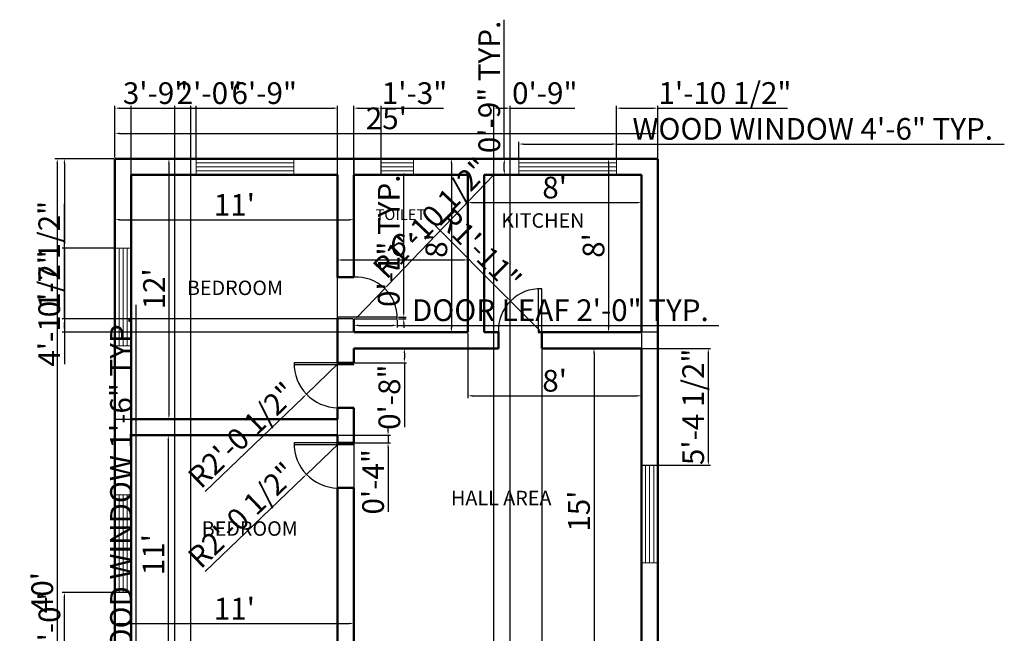
# Model space of a CAD drawing. Units: inches. Extents: x 2490 to 3058, y 1708 to 2351.
# Tile 2 of 2: x 2514 to 3058, y 2012 to 2351. Entities that reach past the tile are written whole.
import ezdxf

# ---------------------------------------------------------------- set-up
doc = ezdxf.new("R2010")
doc.units = ezdxf.units.IN
for name, color, linetype, lineweight in [('A-ANNO-DIMS', 2, 'Continuous', 18), ('A-AREA-IDEN', 7, 'Continuous', 25), ('A-DOOR', 3, 'Continuous', 25), ('A-GLAZ', 4, 'Continuous', 18), ('A-WALL', 7, 'Continuous', 50)]:
    doc.layers.add(name, color=color, linetype=linetype, lineweight=lineweight)
doc.styles.get("Standard").update_dxf_attribs({"font": 'arial.ttf'})
doc.dimstyles.new('ISO-25', dxfattribs={"dimtxt": 12, "dimasz": 2.5, "dimexe": 1.25, "dimexo": 0.625, "dimtad": 1, "dimdec": 1, "dimlunit": 3, "dimtxsty": 'Standard', "dimcen": 2.5, "dimadec": 0, "dimazin": 0, "dimtfac": 1, "dimtdec": 1, "dimtmove": 0, "dimatfit": 3, "dimfxl": 1, "dimarcsym": 0})

# ---------------------------------------------------------------- blocks, each defined once
blk = doc.blocks.new('*D1')
at = {"layer": 'A-ANNO-DIMS', "color": 0, "lineweight": -2, "transparency": 16777216}
for p, q in [((2567.47, 2274.57), (2597.88, 2274.57)), ((2596.63, 2272.07), (2596.63, 2133.07)), ((2567.47, 2130.57), (2597.88, 2130.57))]:
    blk.add_line(p, q, dxfattribs=at)
at = {"layer": 'A-ANNO-DIMS', "color": 0, "transparency": 16777216}
for points in [[(2596.21, 2272.07), (2597.04, 2272.07), (2596.63, 2274.57)], [(2596.21, 2133.07), (2597.04, 2133.07), (2596.63, 2130.57)]]:
    blk.add_solid(points, dxfattribs=at)
at = {"layer": 'Defpoints', "color": 0, "transparency": 16777216}
for p in [(2566.85, 2274.57), (2566.85, 2130.57), (2596.63, 2130.57)]:
    blk.add_point(p, dxfattribs=at)
at = {"layer": 'A-ANNO-DIMS', "color": 0, "transparency": 16777216, "insert": (2589.98, 2202.57), "char_height": 12, "attachment_point": 5, "rotation": 90}
blk.add_mtext("12'", dxfattribs=at)
blk = doc.blocks.new('*D2')
at = {"layer": 'A-ANNO-DIMS', "color": 0, "lineweight": -2, "transparency": 16777216}
for p, q in [((2566.85, 2273.95), (2566.85, 2239.59)), ((2698.85, 2273.95), (2698.85, 2239.59)), ((2569.35, 2240.84), (2696.35, 2240.84))]:
    blk.add_line(p, q, dxfattribs=at)
at = {"layer": 'A-ANNO-DIMS', "color": 0, "transparency": 16777216}
for points in [[(2569.35, 2241.26), (2569.35, 2240.42), (2566.85, 2240.84)], [(2696.35, 2241.26), (2696.35, 2240.42), (2698.85, 2240.84)]]:
    blk.add_solid(points, dxfattribs=at)
at = {"layer": 'Defpoints', "color": 0, "transparency": 16777216}
for p in [(2566.85, 2274.57), (2698.85, 2274.57), (2698.85, 2240.84)]:
    blk.add_point(p, dxfattribs=at)
at = {"layer": 'A-ANNO-DIMS', "color": 0, "transparency": 16777216, "insert": (2632.85, 2247.49), "char_height": 12, "attachment_point": 5}
blk.add_mtext("11'", dxfattribs=at)
blk = doc.blocks.new('*D3')
at = {"layer": 'A-ANNO-DIMS', "color": 0, "lineweight": -2, "transparency": 16777216}
for p, q in [((2689.85, 2209.6), (2689.85, 2219.81)), ((2692.35, 2218.56), (2759.35, 2218.56)), ((2761.85, 2209.6), (2761.85, 2219.81))]:
    blk.add_line(p, q, dxfattribs=at)
at = {"layer": 'A-ANNO-DIMS', "color": 0, "transparency": 16777216}
for points in [[(2692.35, 2218.98), (2692.35, 2218.14), (2689.85, 2218.56)], [(2759.35, 2218.98), (2759.35, 2218.14), (2761.85, 2218.56)]]:
    blk.add_solid(points, dxfattribs=at)
at = {"layer": 'Defpoints', "color": 0, "transparency": 16777216}
for p in [(2761.85, 2218.56), (2689.85, 2208.98), (2761.85, 2208.98)]:
    blk.add_point(p, dxfattribs=at)
at = {"layer": 'A-ANNO-DIMS', "color": 0, "transparency": 16777216, "insert": (2725.85, 2225.31), "char_height": 12, "attachment_point": 5}
blk.add_mtext("6'", dxfattribs=at)
blk = doc.blocks.new('*D4')
at = {"layer": 'A-ANNO-DIMS', "color": 0, "lineweight": -2, "transparency": 16777216}
for p, q in [((2699.47, 2274.57), (2754.03, 2274.57)), ((2752.78, 2272.07), (2752.78, 2181.07)), ((2699.47, 2178.57), (2754.03, 2178.57))]:
    blk.add_line(p, q, dxfattribs=at)
at = {"layer": 'A-ANNO-DIMS', "color": 0, "transparency": 16777216}
for points in [[(2752.37, 2272.07), (2753.2, 2272.07), (2752.78, 2274.57)], [(2752.37, 2181.07), (2753.2, 2181.07), (2752.78, 2178.57)]]:
    blk.add_solid(points, dxfattribs=at)
at = {"layer": 'Defpoints', "color": 0, "transparency": 16777216}
for p in [(2698.85, 2274.57), (2698.85, 2178.57), (2752.78, 2178.57)]:
    blk.add_point(p, dxfattribs=at)
at = {"layer": 'A-ANNO-DIMS', "color": 0, "transparency": 16777216, "insert": (2746.03, 2226.57), "char_height": 12, "attachment_point": 5, "rotation": 90}
blk.add_mtext("8'", dxfattribs=at)
blk = doc.blocks.new('*D5')
at = {"layer": 'A-ANNO-DIMS', "color": 0, "lineweight": -2, "transparency": 16777216}
for p, q in [((2761.85, 2264.95), (2761.85, 2249.05)), ((2857.85, 2264.95), (2857.85, 2249.05)), ((2764.35, 2250.3), (2855.35, 2250.3))]:
    blk.add_line(p, q, dxfattribs=at)
at = {"layer": 'A-ANNO-DIMS', "color": 0, "transparency": 16777216}
for points in [[(2764.35, 2250.71), (2764.35, 2249.88), (2761.85, 2250.3)], [(2855.35, 2250.71), (2855.35, 2249.88), (2857.85, 2250.3)]]:
    blk.add_solid(points, dxfattribs=at)
at = {"layer": 'Defpoints', "color": 0, "transparency": 16777216}
for p in [(2761.85, 2265.57), (2857.85, 2265.57), (2857.85, 2250.3)]:
    blk.add_point(p, dxfattribs=at)
at = {"layer": 'A-ANNO-DIMS', "color": 0, "transparency": 16777216, "insert": (2809.85, 2257.05), "char_height": 12, "attachment_point": 5}
blk.add_mtext("8'", dxfattribs=at)
blk = doc.blocks.new('*D6')
at = {"layer": 'A-ANNO-DIMS', "color": 0, "lineweight": -2, "transparency": 16777216}
for p, q in [((2866.22, 2274.57), (2838.4, 2274.57)), ((2839.65, 2272.07), (2839.65, 2181.07)), ((2866.22, 2178.57), (2838.4, 2178.57))]:
    blk.add_line(p, q, dxfattribs=at)
at = {"layer": 'A-ANNO-DIMS', "color": 0, "transparency": 16777216}
for points in [[(2839.24, 2272.07), (2840.07, 2272.07), (2839.65, 2274.57)], [(2839.24, 2181.07), (2840.07, 2181.07), (2839.65, 2178.57)]]:
    blk.add_solid(points, dxfattribs=at)
at = {"layer": 'Defpoints', "color": 0, "transparency": 16777216}
for p in [(2866.85, 2274.57), (2839.65, 2178.57), (2866.85, 2178.57)]:
    blk.add_point(p, dxfattribs=at)
at = {"layer": 'A-ANNO-DIMS', "color": 0, "transparency": 16777216, "insert": (2832.9, 2226.57), "char_height": 12, "attachment_point": 5, "rotation": 90}
blk.add_mtext("8'", dxfattribs=at)
blk = doc.blocks.new('*D7')
at = {"layer": 'A-ANNO-DIMS', "color": 0, "lineweight": -2, "transparency": 16777216}
for p, q in [((2597.25, 2121.57), (2595.04, 2121.57)), ((2596.29, 2119.07), (2596.29, 1992.07)), ((2597.25, 1989.57), (2595.04, 1989.57))]:
    blk.add_line(p, q, dxfattribs=at)
at = {"layer": 'A-ANNO-DIMS', "color": 0, "transparency": 16777216}
for points in [[(2595.88, 2119.07), (2596.71, 2119.07), (2596.29, 2121.57)], [(2595.88, 1992.07), (2596.71, 1992.07), (2596.29, 1989.57)]]:
    blk.add_solid(points, dxfattribs=at)
at = {"layer": 'Defpoints', "color": 0, "transparency": 16777216}
for p in [(2597.88, 2121.57), (2596.29, 1989.57), (2597.88, 1989.57)]:
    blk.add_point(p, dxfattribs=at)
at = {"layer": 'A-ANNO-DIMS', "color": 0, "transparency": 16777216, "insert": (2589.64, 2055.57), "char_height": 12, "attachment_point": 5, "rotation": 90}
blk.add_mtext("11'", dxfattribs=at)
blk = doc.blocks.new('*D8')
at = {"layer": 'A-ANNO-DIMS', "color": 0, "lineweight": -2, "transparency": 16777216}
for p, q in [((2566.85, 2120.95), (2566.85, 2016.22)), ((2698.85, 2120.95), (2698.85, 2016.22)), ((2569.35, 2017.47), (2696.35, 2017.47))]:
    blk.add_line(p, q, dxfattribs=at)
at = {"layer": 'A-ANNO-DIMS', "color": 0, "transparency": 16777216}
for points in [[(2569.35, 2017.89), (2569.35, 2017.05), (2566.85, 2017.47)], [(2696.35, 2017.89), (2696.35, 2017.05), (2698.85, 2017.47)]]:
    blk.add_solid(points, dxfattribs=at)
at = {"layer": 'Defpoints', "color": 0, "transparency": 16777216}
for p in [(2566.85, 2121.57), (2698.85, 2121.57), (2698.85, 2017.47)]:
    blk.add_point(p, dxfattribs=at)
at = {"layer": 'A-ANNO-DIMS', "color": 0, "transparency": 16777216, "insert": (2632.85, 2024.12), "char_height": 12, "attachment_point": 5}
blk.add_mtext("11'", dxfattribs=at)
blk = doc.blocks.new('*D14')
at = {"layer": 'A-ANNO-DIMS', "color": 0, "lineweight": -2, "transparency": 16777216}
for p, q in [((2847.51, 2169.63), (2830.36, 2169.63)), ((2831.61, 2167.13), (2831.61, 1992.13)), ((2847.51, 1989.63), (2830.36, 1989.63))]:
    blk.add_line(p, q, dxfattribs=at)
at = {"layer": 'A-ANNO-DIMS', "color": 0, "transparency": 16777216}
for points in [[(2831.19, 2167.13), (2832.02, 2167.13), (2831.61, 2169.63)], [(2831.19, 1992.13), (2832.02, 1992.13), (2831.61, 1989.63)]]:
    blk.add_solid(points, dxfattribs=at)
at = {"layer": 'Defpoints', "color": 0, "transparency": 16777216}
for p in [(2848.13, 2169.63), (2831.61, 1989.63), (2848.13, 1989.63)]:
    blk.add_point(p, dxfattribs=at)
at = {"layer": 'A-ANNO-DIMS', "color": 0, "transparency": 16777216, "insert": (2824.86, 2079.63), "char_height": 12, "attachment_point": 5, "rotation": 90}
blk.add_mtext("15'", dxfattribs=at)
blk = doc.blocks.new('*D15')
at = {"layer": 'A-ANNO-DIMS', "color": 0, "lineweight": -2, "transparency": 16777216}
for p, q in [((2761.85, 2177.95), (2761.85, 2142.17)), ((2857.85, 2177.95), (2857.85, 2142.17)), ((2764.35, 2143.42), (2855.35, 2143.42))]:
    blk.add_line(p, q, dxfattribs=at)
at = {"layer": 'A-ANNO-DIMS', "color": 0, "transparency": 16777216}
for points in [[(2764.35, 2143.84), (2764.35, 2143.01), (2761.85, 2143.42)], [(2855.35, 2143.84), (2855.35, 2143.01), (2857.85, 2143.42)]]:
    blk.add_solid(points, dxfattribs=at)
at = {"layer": 'Defpoints', "color": 0, "transparency": 16777216}
for p in [(2761.85, 2178.57), (2857.85, 2178.57), (2857.85, 2143.42)]:
    blk.add_point(p, dxfattribs=at)
at = {"layer": 'A-ANNO-DIMS', "color": 0, "transparency": 16777216, "insert": (2809.85, 2150.17), "char_height": 12, "attachment_point": 5}
blk.add_mtext("8'", dxfattribs=at)
blk = doc.blocks.new('Window - Wood Frame 36 in. Wide plan')
for p, q in [((0, 6), (0, 0)), ((0, 4.5), (36, 4.5)), ((36, 6), (36, 0)), ((0, 3), (36, 3)), ((0, 1.5), (36, 1.5))]:
    blk.add_line(p, q)
blk = doc.blocks.new('*D21')
at = {"layer": 'A-ANNO-DIMS', "color": 0, "lineweight": -2, "transparency": 16777216}
for p, q in [((2566.85, 2275.2), (2566.85, 2289.82)), ((2569.35, 2288.57), (2864.35, 2288.57)), ((2866.85, 2275.2), (2866.85, 2289.82))]:
    blk.add_line(p, q, dxfattribs=at)
at = {"layer": 'A-ANNO-DIMS', "color": 0, "transparency": 16777216}
for points in [[(2569.35, 2288.99), (2569.35, 2288.16), (2566.85, 2288.57)], [(2864.35, 2288.99), (2864.35, 2288.16), (2866.85, 2288.57)]]:
    blk.add_solid(points, dxfattribs=at)
at = {"layer": 'Defpoints', "color": 0, "transparency": 16777216}
for p in [(2866.85, 2288.57), (2566.85, 2274.57), (2866.85, 2274.57)]:
    blk.add_point(p, dxfattribs=at)
at = {"layer": 'A-ANNO-DIMS', "color": 0, "transparency": 16777216, "insert": (2716.85, 2295.33), "char_height": 12, "attachment_point": 5}
blk.add_mtext("25'", dxfattribs=at)
blk = doc.blocks.new('*D22')
at = {"layer": 'A-ANNO-DIMS', "color": 0, "lineweight": -2, "transparency": 16777216}
for p, q in [((2566.22, 2274.57), (2533.68, 2274.57)), ((2534.93, 2272.07), (2534.93, 1797.07)), ((2566.22, 1794.57), (2533.68, 1794.57))]:
    blk.add_line(p, q, dxfattribs=at)
at = {"layer": 'A-ANNO-DIMS', "color": 0, "transparency": 16777216}
for points in [[(2534.51, 2272.07), (2535.35, 2272.07), (2534.93, 2274.57)], [(2534.51, 1797.07), (2535.35, 1797.07), (2534.93, 1794.57)]]:
    blk.add_solid(points, dxfattribs=at)
at = {"layer": 'Defpoints', "color": 0, "transparency": 16777216}
for p in [(2566.85, 2274.57), (2534.93, 1794.57), (2566.85, 1794.57)]:
    blk.add_point(p, dxfattribs=at)
at = {"layer": 'A-ANNO-DIMS', "color": 0, "transparency": 16777216, "insert": (2528.18, 2034.57), "char_height": 12, "attachment_point": 5, "rotation": 90}
blk.add_mtext("40'", dxfattribs=at)
blk = doc.blocks.new('DOOR-LEAF-24IN')
for p, q in [((24, 1), (0, 1)), ((0, 0), (24, 0)), ((24, 0), (24, 1))]:
    blk.add_line(p, q)
blk = doc.blocks.new('*D24')
at = {"layer": 'A-ANNO-DIMS', "color": 0, "lineweight": -2, "transparency": 16777216}
for p, q in [((2790.13, 2275.2), (2790.13, 2283.92)), ((2792.63, 2282.67), (2841.63, 2282.67)), ((2844.13, 2275.2), (2844.13, 2283.92)), ((2844.13, 2282.67), (3058.39, 2282.67))]:
    blk.add_line(p, q, dxfattribs=at)
at = {"layer": 'A-ANNO-DIMS', "color": 0, "transparency": 16777216}
for points in [[(2792.63, 2283.09), (2792.63, 2282.25), (2790.13, 2282.67)], [(2841.63, 2283.09), (2841.63, 2282.25), (2844.13, 2282.67)]]:
    blk.add_solid(points, dxfattribs=at)
at = {"layer": 'Defpoints', "color": 0, "transparency": 16777216}
for p in [(2844.13, 2282.67), (2790.13, 2274.57), (2844.13, 2274.57)]:
    blk.add_point(p, dxfattribs=at)
at = {"layer": 'A-ANNO-DIMS', "color": 0, "transparency": 16777216, "insert": (2952.51, 2289.5), "char_height": 12, "attachment_point": 5}
blk.add_mtext('WOOD WINDOW 4\'-6" TYP.', dxfattribs=at)
blk = doc.blocks.new('*D25')
at = {"layer": 'A-ANNO-DIMS', "color": 0, "lineweight": -2, "transparency": 16777216}
for p, q in [((2782.03, 2274.57), (2782.03, 2351.47)), ((2789.5, 2274.57), (2780.78, 2274.57)), ((2782.03, 2268.07), (2782.03, 2272.07)), ((2789.5, 2265.57), (2780.78, 2265.57))]:
    blk.add_line(p, q, dxfattribs=at)
at = {"layer": 'A-ANNO-DIMS', "color": 0, "transparency": 16777216}
for points in [[(2781.61, 2272.07), (2782.44, 2272.07), (2782.03, 2274.57)], [(2781.61, 2268.07), (2782.44, 2268.07), (2782.03, 2265.57)]]:
    blk.add_solid(points, dxfattribs=at)
at = {"layer": 'Defpoints', "color": 0, "transparency": 16777216}
for p in [(2782.03, 2274.57), (2790.13, 2274.57), (2790.13, 2265.57)]:
    blk.add_point(p, dxfattribs=at)
at = {"layer": 'A-ANNO-DIMS', "color": 0, "transparency": 16777216, "insert": (2775.28, 2314.27), "char_height": 12, "attachment_point": 5, "rotation": 90}
blk.add_mtext('0\'-9" TYP.', dxfattribs=at)
blk = doc.blocks.new('*D26')
at = {"layer": 'A-ANNO-DIMS', "color": 0, "lineweight": -2, "transparency": 16777216}
for p, q in [((2578.55, 1979.48), (2578.55, 2193.75)), ((2576.47, 1979.48), (2579.8, 1979.48)), ((2578.55, 1963.98), (2578.55, 1976.98)), ((2576.47, 1961.48), (2579.8, 1961.48))]:
    blk.add_line(p, q, dxfattribs=at)
at = {"layer": 'A-ANNO-DIMS', "color": 0, "transparency": 16777216}
for points in [[(2578.13, 1976.98), (2578.97, 1976.98), (2578.55, 1979.48)], [(2578.13, 1963.98), (2578.97, 1963.98), (2578.55, 1961.48)]]:
    blk.add_solid(points, dxfattribs=at)
at = {"layer": 'Defpoints', "color": 0, "transparency": 16777216}
for p in [(2575.85, 1979.48), (2578.55, 1979.48), (2575.85, 1961.48)]:
    blk.add_point(p, dxfattribs=at)
at = {"layer": 'A-ANNO-DIMS', "color": 0, "transparency": 16777216, "insert": (2571.72, 2087.86), "char_height": 12, "attachment_point": 5, "rotation": 90}
blk.add_mtext('WOOD WINDOW 1\'-6" TYP.', dxfattribs=at)
blk = doc.blocks.new('*D28')
at = {"layer": 'A-ANNO-DIMS', "color": 0, "lineweight": -2, "transparency": 16777216}
for p, q in [((2698.85, 2185.35), (2698.85, 2181.13)), ((2701.35, 2182.38), (2720.35, 2182.38)), ((2722.85, 2185.35), (2722.85, 2181.13)), ((2722.85, 2182.38), (2900.68, 2182.38))]:
    blk.add_line(p, q, dxfattribs=at)
at = {"layer": 'A-ANNO-DIMS', "color": 0, "transparency": 16777216}
for points in [[(2701.35, 2182.8), (2701.35, 2181.96), (2698.85, 2182.38)], [(2720.35, 2182.8), (2720.35, 2181.96), (2722.85, 2182.38)]]:
    blk.add_solid(points, dxfattribs=at)
at = {"layer": 'Defpoints', "color": 0, "transparency": 16777216}
for p in [(2698.85, 2185.98), (2722.85, 2185.98), (2722.85, 2182.38)]:
    blk.add_point(p, dxfattribs=at)
at = {"layer": 'A-ANNO-DIMS', "color": 0, "transparency": 16777216, "insert": (2813.01, 2189.21), "char_height": 12, "attachment_point": 5}
blk.add_mtext('DOOR LEAF 2\'-0" TYP.', dxfattribs=at)
blk = doc.blocks.new('*D29')
at = {"layer": 'A-ANNO-DIMS', "color": 0, "lineweight": -2, "transparency": 16777216}
for p, q in [((2726.45, 2189.48), (2726.45, 2266.37)), ((2723.47, 2186.98), (2727.7, 2186.98)), ((2723.47, 2185.98), (2727.7, 2185.98)), ((2726.45, 2185.98), (2726.45, 2186.98)), ((2726.45, 2183.48), (2726.45, 2180.98))]:
    blk.add_line(p, q, dxfattribs=at)
at = {"layer": 'A-ANNO-DIMS', "color": 0, "transparency": 16777216}
for points in [[(2726.03, 2189.48), (2726.87, 2189.48), (2726.45, 2186.98)], [(2726.03, 2183.48), (2726.87, 2183.48), (2726.45, 2185.98)]]:
    blk.add_solid(points, dxfattribs=at)
at = {"layer": 'Defpoints', "color": 0, "transparency": 16777216}
for p in [(2722.85, 2186.98), (2722.85, 2185.98), (2726.45, 2186.98)]:
    blk.add_point(p, dxfattribs=at)
at = {"layer": 'A-ANNO-DIMS', "color": 0, "transparency": 16777216, "insert": (2719.7, 2229.18), "char_height": 12, "attachment_point": 5, "rotation": 90}
blk.add_mtext('0\'-1" TYP.', dxfattribs=at)
blk = doc.blocks.new('*D33')
at = {"layer": 'A-ANNO-DIMS', "color": 0, "lineweight": -2, "transparency": 16777216}
for p, q in [((2608.85, 1990.2), (2608.85, 2303.77)), ((2611.35, 2302.52), (2687.35, 2302.52)), ((2689.85, 1990.2), (2689.85, 2303.77))]:
    blk.add_line(p, q, dxfattribs=at)
at = {"layer": 'A-ANNO-DIMS', "color": 0, "transparency": 16777216}
for points in [[(2611.35, 2302.94), (2611.35, 2302.1), (2608.85, 2302.52)], [(2687.35, 2302.94), (2687.35, 2302.1), (2689.85, 2302.52)]]:
    blk.add_solid(points, dxfattribs=at)
at = {"layer": 'Defpoints', "color": 0, "transparency": 16777216}
for p in [(2689.85, 2302.52), (2608.85, 1989.57), (2689.85, 1989.57)]:
    blk.add_point(p, dxfattribs=at)
at = {"layer": 'A-ANNO-DIMS', "color": 0, "transparency": 16777216, "insert": (2649.35, 2309.27), "char_height": 12, "attachment_point": 5}
blk.add_mtext('6\'-9"', dxfattribs=at)
blk = doc.blocks.new('*D34')
at = {"layer": 'A-ANNO-DIMS', "color": 0, "lineweight": -2, "transparency": 16777216}
for p, q in [((2698.85, 2266.2), (2698.85, 2303.77)), ((2701.35, 2302.52), (2711.41, 2302.52)), ((2713.91, 2266.2), (2713.91, 2303.77)), ((2713.91, 2302.52), (2748.42, 2302.52))]:
    blk.add_line(p, q, dxfattribs=at)
at = {"layer": 'A-ANNO-DIMS', "color": 0, "transparency": 16777216}
for points in [[(2701.35, 2302.94), (2701.35, 2302.1), (2698.85, 2302.52)], [(2711.41, 2302.94), (2711.41, 2302.1), (2713.91, 2302.52)]]:
    blk.add_solid(points, dxfattribs=at)
at = {"layer": 'Defpoints', "color": 0, "transparency": 16777216}
for p in [(2713.91, 2302.52), (2698.85, 2265.57), (2713.91, 2265.57)]:
    blk.add_point(p, dxfattribs=at)
at = {"layer": 'A-ANNO-DIMS', "color": 0, "transparency": 16777216, "insert": (2732.42, 2309.28), "char_height": 12, "attachment_point": 5}
blk.add_mtext('1\'-3"', dxfattribs=at)
blk = doc.blocks.new('*D35')
at = {"layer": 'A-ANNO-DIMS', "color": 0, "lineweight": -2, "transparency": 16777216}
for p, q in [((2844.13, 2275.2), (2844.13, 2303.77)), ((2846.63, 2302.52), (2864.35, 2302.52)), ((2866.85, 2275.2), (2866.85, 2303.77)), ((2866.85, 2302.52), (2938.65, 2302.52))]:
    blk.add_line(p, q, dxfattribs=at)
at = {"layer": 'A-ANNO-DIMS', "color": 0, "transparency": 16777216}
for points in [[(2846.63, 2302.94), (2846.63, 2302.1), (2844.13, 2302.52)], [(2864.35, 2302.94), (2864.35, 2302.1), (2866.85, 2302.52)]]:
    blk.add_solid(points, dxfattribs=at)
at = {"layer": 'Defpoints', "color": 0, "transparency": 16777216}
for p in [(2866.85, 2302.52), (2844.13, 2274.57), (2866.85, 2274.57)]:
    blk.add_point(p, dxfattribs=at)
at = {"layer": 'A-ANNO-DIMS', "color": 0, "transparency": 16777216, "insert": (2904, 2309.35), "char_height": 12, "attachment_point": 5}
blk.add_mtext('1\'-10 1/2"', dxfattribs=at)
blk = doc.blocks.new('*D36')
at = {"layer": 'A-ANNO-DIMS', "color": 0, "lineweight": -2, "transparency": 16777216}
for p, q in [((2802.74, 2168.95), (2802.74, 1718.25)), ((2857.85, 2168.95), (2857.85, 1718.25)), ((2805.24, 1719.5), (2855.35, 1719.5))]:
    blk.add_line(p, q, dxfattribs=at)
at = {"layer": 'A-ANNO-DIMS', "color": 0, "transparency": 16777216}
for points in [[(2805.24, 1719.92), (2805.24, 1719.08), (2802.74, 1719.5)], [(2855.35, 1719.92), (2855.35, 1719.08), (2857.85, 1719.5)]]:
    blk.add_solid(points, dxfattribs=at)
at = {"layer": 'Defpoints', "color": 0, "transparency": 16777216}
for p in [(2802.74, 2169.57), (2857.85, 2169.57), (2857.85, 1719.5)]:
    blk.add_point(p, dxfattribs=at)
at = {"layer": 'A-ANNO-DIMS', "color": 0, "transparency": 16777216, "insert": (2830.3, 1726.12), "char_height": 12, "attachment_point": 5}
blk.add_mtext('4\'-7"', dxfattribs=at)
blk = doc.blocks.new('*D37')
at = {"layer": 'A-ANNO-DIMS', "color": 0, "lineweight": -2, "transparency": 16777216}
for p, q in [((2538.9, 2185.98), (2538.9, 2249.59)), ((2698.22, 2185.98), (2537.65, 2185.98)), ((2538.9, 2181.07), (2538.9, 2183.48)), ((2698.22, 2178.57), (2537.65, 2178.57))]:
    blk.add_line(p, q, dxfattribs=at)
at = {"layer": 'A-ANNO-DIMS', "color": 0, "transparency": 16777216}
for points in [[(2538.48, 2183.48), (2539.32, 2183.48), (2538.9, 2185.98)], [(2538.48, 2181.07), (2539.32, 2181.07), (2538.9, 2178.57)]]:
    blk.add_solid(points, dxfattribs=at)
at = {"layer": 'Defpoints', "color": 0, "transparency": 16777216}
for p in [(2538.9, 2185.98), (2698.85, 2185.98), (2698.85, 2178.57)]:
    blk.add_point(p, dxfattribs=at)
at = {"layer": 'A-ANNO-DIMS', "color": 0, "transparency": 16777216, "insert": (2532.07, 2219.03), "char_height": 12, "attachment_point": 5, "rotation": 90}
blk.add_mtext('0\'-7 1/2"', dxfattribs=at)
blk = doc.blocks.new('*D40')
at = {"layer": 'A-ANNO-DIMS', "color": 0, "lineweight": -2, "transparency": 16777216}
for p, q in [((2575.85, 1990.2), (2575.85, 2303.77)), ((2578.35, 2302.52), (2597.35, 2302.52)), ((2599.85, 1990.2), (2599.85, 2303.77)), ((2599.85, 2302.52), (2635.7, 2302.52))]:
    blk.add_line(p, q, dxfattribs=at)
at = {"layer": 'A-ANNO-DIMS', "color": 0, "transparency": 16777216}
for points in [[(2578.35, 2302.94), (2578.35, 2302.1), (2575.85, 2302.52)], [(2597.35, 2302.94), (2597.35, 2302.1), (2599.85, 2302.52)]]:
    blk.add_solid(points, dxfattribs=at)
at = {"layer": 'Defpoints', "color": 0, "transparency": 16777216}
for p in [(2599.85, 2302.52), (2575.85, 1989.57), (2599.85, 1989.57)]:
    blk.add_point(p, dxfattribs=at)
at = {"layer": 'A-ANNO-DIMS', "color": 0, "transparency": 16777216, "insert": (2619.03, 2309.27), "char_height": 12, "attachment_point": 5}
blk.add_mtext('2\'-0"', dxfattribs=at)
blk = doc.blocks.new('*D41')
at = {"layer": 'A-ANNO-DIMS', "color": 0, "lineweight": -2, "transparency": 16777216}
for p, q in [((2566.85, 2275.2), (2566.85, 2303.77)), ((2569.35, 2302.52), (2609.21, 2302.52)), ((2611.71, 2275.2), (2611.71, 2303.77))]:
    blk.add_line(p, q, dxfattribs=at)
at = {"layer": 'A-ANNO-DIMS', "color": 0, "transparency": 16777216}
for points in [[(2569.35, 2302.94), (2569.35, 2302.1), (2566.85, 2302.52)], [(2609.21, 2302.94), (2609.21, 2302.1), (2611.71, 2302.52)]]:
    blk.add_solid(points, dxfattribs=at)
at = {"layer": 'Defpoints', "color": 0, "transparency": 16777216}
for p in [(2611.71, 2302.52), (2566.85, 2274.57), (2611.71, 2274.57)]:
    blk.add_point(p, dxfattribs=at)
at = {"layer": 'A-ANNO-DIMS', "color": 0, "transparency": 16777216, "insert": (2589.28, 2309.28), "char_height": 12, "attachment_point": 5}
blk.add_mtext('3\'-9"', dxfattribs=at)
blk = doc.blocks.new('*D42')
at = {"layer": 'A-ANNO-DIMS', "color": 0, "lineweight": -2, "transparency": 16777216}
for p, q in [((2566.22, 2274.57), (2537.65, 2274.57)), ((2538.9, 2272.07), (2538.9, 2227.55)), ((2566.22, 2225.05), (2537.65, 2225.05)), ((2538.9, 2225.05), (2538.9, 2160.95))]:
    blk.add_line(p, q, dxfattribs=at)
at = {"layer": 'A-ANNO-DIMS', "color": 0, "transparency": 16777216}
for points in [[(2538.48, 2272.07), (2539.32, 2272.07), (2538.9, 2274.57)], [(2538.48, 2227.55), (2539.32, 2227.55), (2538.9, 2225.05)]]:
    blk.add_solid(points, dxfattribs=at)
at = {"layer": 'Defpoints', "color": 0, "transparency": 16777216}
for p in [(2566.85, 2274.57), (2538.9, 2225.05), (2566.85, 2225.05)]:
    blk.add_point(p, dxfattribs=at)
at = {"layer": 'A-ANNO-DIMS', "color": 0, "transparency": 16777216, "insert": (2532.07, 2191.75), "char_height": 12, "attachment_point": 5, "rotation": 90}
blk.add_mtext('4\'-1 1/2"', dxfattribs=at)
blk = doc.blocks.new('*D43')
at = {"layer": 'A-ANNO-DIMS', "color": 0, "lineweight": -2, "transparency": 16777216}
for p, q in [((2575.22, 2034.57), (2537.65, 2034.57)), ((2538.9, 2001.07), (2538.9, 2032.07)), ((2575.22, 1998.57), (2537.65, 1998.57))]:
    blk.add_line(p, q, dxfattribs=at)
at = {"layer": 'A-ANNO-DIMS', "color": 0, "transparency": 16777216}
for points in [[(2538.48, 2032.07), (2539.32, 2032.07), (2538.9, 2034.57)], [(2538.48, 2001.07), (2539.32, 2001.07), (2538.9, 1998.57)]]:
    blk.add_solid(points, dxfattribs=at)
at = {"layer": 'Defpoints', "color": 0, "transparency": 16777216}
for p in [(2538.9, 2034.57), (2575.85, 2034.57), (2575.85, 1998.57)]:
    blk.add_point(p, dxfattribs=at)
at = {"layer": 'A-ANNO-DIMS', "color": 0, "transparency": 16777216, "insert": (2532.14, 2016.57), "char_height": 12, "attachment_point": 5, "rotation": 90}
blk.add_mtext('3\'-0"', dxfattribs=at)
blk = doc.blocks.new('*D46')
at = {"layer": 'A-ANNO-DIMS', "color": 0, "lineweight": -2, "transparency": 16777216}
for p, q in [((2858.47, 2169.57), (2896.05, 2169.57)), ((2894.8, 2167.07), (2894.8, 2107.54)), ((2858.47, 2105.04), (2896.05, 2105.04))]:
    blk.add_line(p, q, dxfattribs=at)
at = {"layer": 'A-ANNO-DIMS', "color": 0, "transparency": 16777216}
for points in [[(2894.38, 2167.07), (2895.22, 2167.07), (2894.8, 2169.57)], [(2894.38, 2107.54), (2895.22, 2107.54), (2894.8, 2105.04)]]:
    blk.add_solid(points, dxfattribs=at)
at = {"layer": 'Defpoints', "color": 0, "transparency": 16777216}
for p in [(2857.85, 2169.57), (2857.85, 2105.04), (2894.8, 2105.04)]:
    blk.add_point(p, dxfattribs=at)
at = {"layer": 'A-ANNO-DIMS', "color": 0, "transparency": 16777216, "insert": (2887.97, 2137.31), "char_height": 12, "attachment_point": 5, "rotation": 90}
blk.add_mtext('5\'-4 1/2"', dxfattribs=at)
blk = doc.blocks.new('*D48')
at = {"layer": 'A-ANNO-DIMS', "color": 0, "lineweight": -2, "transparency": 16777216}
for p, q in [((2699.47, 2169.57), (2728.05, 2169.57)), ((2726.8, 2167.07), (2726.8, 2164.24)), ((2699.47, 2161.74), (2728.05, 2161.74)), ((2726.8, 2161.74), (2726.8, 2126.09))]:
    blk.add_line(p, q, dxfattribs=at)
at = {"layer": 'A-ANNO-DIMS', "color": 0, "transparency": 16777216}
for points in [[(2726.38, 2167.07), (2727.22, 2167.07), (2726.8, 2169.57)], [(2726.38, 2164.24), (2727.22, 2164.24), (2726.8, 2161.74)]]:
    blk.add_solid(points, dxfattribs=at)
at = {"layer": 'Defpoints', "color": 0, "transparency": 16777216}
for p in [(2698.85, 2169.57), (2698.85, 2161.74), (2726.8, 2161.74)]:
    blk.add_point(p, dxfattribs=at)
at = {"layer": 'A-ANNO-DIMS', "color": 0, "transparency": 16777216, "insert": (2720.05, 2142.66), "char_height": 12, "attachment_point": 5, "rotation": 90}
blk.add_mtext('0\'-8"', dxfattribs=at)
blk = doc.blocks.new('*D49')
at = {"layer": 'A-ANNO-DIMS', "color": 0, "lineweight": -2, "transparency": 16777216}
for p, q in [((2717.8, 2124.07), (2717.8, 2126.57)), ((2690.47, 2121.57), (2719.05, 2121.57)), ((2690.47, 2117.42), (2719.05, 2117.42)), ((2717.8, 2121.57), (2717.8, 2117.42)), ((2717.8, 2114.92), (2717.8, 2079.27))]:
    blk.add_line(p, q, dxfattribs=at)
at = {"layer": 'A-ANNO-DIMS', "color": 0, "transparency": 16777216}
for points in [[(2717.38, 2124.07), (2718.22, 2124.07), (2717.8, 2121.57)], [(2717.38, 2114.92), (2718.22, 2114.92), (2717.8, 2117.42)]]:
    blk.add_solid(points, dxfattribs=at)
at = {"layer": 'Defpoints', "color": 0, "transparency": 16777216}
for p in [(2689.85, 2121.57), (2689.85, 2117.42), (2717.8, 2117.42)]:
    blk.add_point(p, dxfattribs=at)
at = {"layer": 'A-ANNO-DIMS', "color": 0, "transparency": 16777216, "insert": (2711.05, 2095.84), "char_height": 12, "attachment_point": 5, "rotation": 90}
blk.add_mtext('0\'-4"', dxfattribs=at)
blk = doc.blocks.new('*D51')
at = {"layer": 'A-ANNO-DIMS', "color": 0, "lineweight": -2, "transparency": 16777216}
for p, q in [((2776.33, 1988.2), (2776.33, 2303.77)), ((2778.83, 2302.52), (2782.83, 2302.52)), ((2785.33, 1988.2), (2785.33, 2303.77)), ((2785.33, 2302.52), (2820.98, 2302.52))]:
    blk.add_line(p, q, dxfattribs=at)
at = {"layer": 'A-ANNO-DIMS', "color": 0, "transparency": 16777216}
for points in [[(2778.83, 2302.94), (2778.83, 2302.1), (2776.33, 2302.52)], [(2782.83, 2302.94), (2782.83, 2302.1), (2785.33, 2302.52)]]:
    blk.add_solid(points, dxfattribs=at)
at = {"layer": 'Defpoints', "color": 0, "transparency": 16777216}
for p in [(2785.33, 2302.52), (2776.33, 1987.57), (2785.33, 1987.57)]:
    blk.add_point(p, dxfattribs=at)
at = {"layer": 'A-ANNO-DIMS', "color": 0, "transparency": 16777216, "insert": (2804.41, 2309.27), "char_height": 12, "attachment_point": 5}
blk.add_mtext('0\'-9"', dxfattribs=at)
blk = doc.blocks.new('*D56')
at = {"layer": 'A-ANNO-DIMS', "color": 0, "lineweight": -2, "transparency": 16777216}
for p, q in [((2690.35, 2116.92), (2672.67, 2099.95)), ((2616.7, 2046.21), (2670.87, 2098.21))]:
    blk.add_line(p, q, dxfattribs=at)
at = {"layer": 'A-ANNO-DIMS', "color": 0, "transparency": 16777216}
blk.add_solid([(2670.58, 2098.51), (2671.16, 2097.91), (2672.67, 2099.95)], dxfattribs=at)
at = {"layer": 'Defpoints', "color": 0, "transparency": 16777216}
for p in [(2690.35, 2116.92), (2672.67, 2099.95)]:
    blk.add_point(p, dxfattribs=at)
at = {"layer": 'A-ANNO-DIMS', "color": 0, "transparency": 16777216, "insert": (2638.15, 2076.27), "char_height": 12, "attachment_point": 5, "rotation": 43.831}
blk.add_mtext('R2\'-0 1/2"', dxfattribs=at)
blk = doc.blocks.new('*D57')
at = {"layer": 'A-ANNO-DIMS', "color": 0, "lineweight": -2, "transparency": 16777216}
for p, q in [((2690.28, 2161.24), (2672.68, 2144.29)), ((2616.77, 2090.48), (2670.87, 2142.56))]:
    blk.add_line(p, q, dxfattribs=at)
at = {"layer": 'A-ANNO-DIMS', "color": 0, "transparency": 16777216}
blk.add_solid([(2670.58, 2142.86), (2671.16, 2142.26), (2672.68, 2144.29)], dxfattribs=at)
at = {"layer": 'Defpoints', "color": 0, "transparency": 16777216}
for p in [(2690.28, 2161.24), (2672.68, 2144.29)]:
    blk.add_point(p, dxfattribs=at)
at = {"layer": 'A-ANNO-DIMS', "color": 0, "transparency": 16777216, "insert": (2638.18, 2120.57), "char_height": 12, "attachment_point": 5, "rotation": 43.9044}
blk.add_mtext('R2\'-0 1/2"', dxfattribs=at)
blk = doc.blocks.new('*D58')
at = {"layer": 'A-ANNO-DIMS', "color": 0, "lineweight": -2, "transparency": 16777216}
for p, q in [((2743.78, 2237.54), (2783.7, 2197.62)), ((2801.74, 2179.57), (2785.47, 2195.85))]:
    blk.add_line(p, q, dxfattribs=at)
at = {"layer": 'A-ANNO-DIMS', "color": 0, "transparency": 16777216}
blk.add_solid([(2783.99, 2197.91), (2783.4, 2197.32), (2785.47, 2195.85)], dxfattribs=at)
at = {"layer": 'Defpoints', "color": 0, "transparency": 16777216}
for p in [(2785.47, 2195.85), (2801.74, 2179.57)]:
    blk.add_point(p, dxfattribs=at)
at = {"layer": 'A-ANNO-DIMS', "color": 0, "transparency": 16777216, "insert": (2767.56, 2223.16), "char_height": 12, "attachment_point": 5, "rotation": 314.9994}
blk.add_mtext('R1\'-11"', dxfattribs=at)
blk = doc.blocks.new('*D59')
at = {"layer": 'A-ANNO-DIMS', "color": 0, "lineweight": -2, "transparency": 16777216}
for p, q in [((2776.05, 2265.51), (2717.64, 2204.56)), ((2700.31, 2186.48), (2715.91, 2202.76))]:
    blk.add_line(p, q, dxfattribs=at)
at = {"layer": 'A-ANNO-DIMS', "color": 0, "transparency": 16777216}
blk.add_solid([(2717.34, 2204.85), (2717.94, 2204.27), (2715.91, 2202.76)], dxfattribs=at)
at = {"layer": 'Defpoints', "color": 0, "transparency": 16777216}
for p in [(2715.91, 2202.76), (2700.31, 2186.48)]:
    blk.add_point(p, dxfattribs=at)
at = {"layer": 'A-ANNO-DIMS', "color": 0, "transparency": 16777216, "insert": (2742.78, 2240.66), "char_height": 12, "attachment_point": 5, "rotation": 46.2181}
blk.add_mtext('R1\'-10 1/2"', dxfattribs=at)

msp = doc.modelspace()

# ---------------------------------------------------------------- linework, layer by layer
at = {"layer": 'A-DOOR'}
for p, q in [((2802.74, 2202.57), (2800.74, 2202.57)), ((2800.74, 2202.57), (2800.74, 2178.57)), ((2802.74, 2178.57), (2802.74, 2202.57)), ((2698.85, 2186.98), (2689.85, 2186.98)), ((2689.85, 2186.98), (2689.85, 2185.98)), ((2689.85, 2161.74), (2665.85, 2161.74)), ((2665.85, 2161.74), (2665.85, 2160.74)), ((2665.85, 2160.74), (2698.85, 2160.74)), ((2698.85, 2160.74), (2698.85, 2161.74)), ((2698.85, 2116.42), (2698.85, 2117.42)), ((2689.85, 2116.42), (2698.85, 2116.42))]:
    msp.add_line(p, q, dxfattribs=at)
for centre, radius, start, end in [((2700.31, 2186.48), 22.55, 358.7293, 93.7084), ((2801.74, 2179.57), 23.02, 87.5104, 182.4896), ((2690.28, 2161.24), 24.44, 178.8278, 268.9787), ((2690.35, 2116.92), 24.51, 178.8309, 268.8309)]:
    msp.add_arc(centre, radius, start, end, dxfattribs=at)
at = {"layer": 'A-WALL'}
for p, q in [((2566.85, 2274.57), (2866.85, 2274.57)), ((2566.85, 1794.57), (2566.85, 2274.57)), ((2866.85, 2274.57), (2866.85, 1794.57)), ((2575.85, 2265.57), (2689.85, 2265.57)), ((2575.85, 1998.57), (2575.85, 2265.57)), ((2689.85, 2208.98), (2689.85, 2265.57)), ((2698.85, 2265.57), (2761.85, 2265.57)), ((2698.85, 2208.98), (2698.85, 2265.57)), ((2761.85, 2178.57), (2761.85, 2265.57)), ((2770.85, 2178.57), (2770.85, 2265.57)), ((2770.85, 2265.57), (2857.85, 2265.57)), ((2857.85, 2265.57), (2857.85, 2178.57)), ((2689.85, 2208.98), (2698.85, 2208.98)), ((2689.85, 2169.57), (2689.85, 2185.98)), ((2698.85, 2178.57), (2698.85, 2185.98)), ((2698.85, 2178.57), (2761.85, 2178.57)), ((2770.85, 2178.57), (2778.74, 2178.57)), ((2778.74, 2178.57), (2778.74, 2169.57)), ((2800.74, 2178.57), (2857.85, 2178.57)), ((2802.74, 2178.57), (2802.74, 2169.57)), ((2689.85, 2169.57), (2689.85, 2168.57)), ((2689.85, 2168.57), (2689.85, 2161.74)), ((2698.85, 2169.57), (2770.85, 2169.57)), ((2698.85, 2161.74), (2698.85, 2169.57)), ((2770.85, 2169.57), (2778.74, 2169.57)), ((2802.74, 2169.57), (2857.85, 2169.57)), ((2857.85, 2169.57), (2857.85, 1998.57)), ((2698.85, 2161.74), (2689.85, 2161.74)), ((2698.85, 2161.74), (2689.85, 2161.74)), ((2689.85, 2136.8), (2698.85, 2136.8)), ((2689.85, 2130.57), (2689.85, 2136.8)), ((2698.85, 2117.42), (2698.85, 2136.8)), ((2575.85, 2130.57), (2689.85, 2130.57)), ((2575.85, 2121.57), (2689.85, 2121.57)), ((2689.85, 2116.42), (2689.85, 2121.57)), ((2689.85, 2117.42), (2698.85, 2117.42)), ((2689.85, 2092.42), (2698.85, 2092.42)), ((2689.85, 1998.57), (2689.85, 2092.42)), ((2698.85, 1984.57), (2698.85, 2092.42))]:
    msp.add_line(p, q, dxfattribs=at)

# ---------------------------------------------------------------- block references
at = {"layer": 'A-DOOR'}
msp.add_blockref('DOOR-LEAF-24IN', (2698.85, 2185.98), dxfattribs=at)
at = {"layer": 'A-DOOR', "rotation": 180}
msp.add_blockref('DOOR-LEAF-24IN', (2689.85, 2117.42), dxfattribs=at)
at = {"layer": 'A-GLAZ', "xscale": 1.5, "yscale": 1.5}
for p in [(2611.71, 2265.57), (2790.13, 2265.57)]:
    msp.add_blockref('Window - Wood Frame 36 in. Wide plan', p, dxfattribs=at)
at = {"layer": 'A-GLAZ', "yscale": 1.5}
for p, xscale, rotation in [((2731.91, 2274.57), 0.5, 180), ((2575.85, 2171.05), 1.5, 90), ((2866.85, 2051.04), 1.5, 90), ((2575.85, 2034.57), 1.5, 90)]:
    msp.add_blockref('Window - Wood Frame 36 in. Wide plan', p, dxfattribs=dict(at, xscale=xscale, rotation=rotation))

# ---------------------------------------------------------------- texts
at = {"layer": 'A-AREA-IDEN', "attachment_point": 1}
for s, width, heights, insert, char_height in [('TOILET', 31.2754, [6.21], (2710.83, 2246.64), 6), ('KITCHEN', 84.6482, [0], (2780.3, 2244.39), 8), ('BEDROOM', 0.8182, [0], (2606.62, 2207.14), 8), ('HALL AREA', 84.6482, [0], (2752.57, 2090.89), 8), ('BEDROOM', 0.8182, [0], (2614.8, 2073.98), 8)]:
    msp.add_mtext_dynamic_manual_height_columns(s, width=width, gutter_width=12.5, heights=heights, dxfattribs=dict(at, insert=insert, char_height=char_height))

# ---------------------------------------------------------------- dimensions: what is measured, and where the dimension line sits
at = {"layer": 'A-ANNO-DIMS'}
for base, p1, p2, text, picture, middle in [((2782.03, 2274.57), (2790.13, 2265.57), (2790.13, 2274.57), '<> TYP.', '*D25', (2775.28, 2314.27)), ((2726.45, 2186.98), (2722.85, 2185.98), (2722.85, 2186.98), '<> TYP.', '*D29', (2719.7, 2229.18)), ((2578.55, 1979.48), (2575.85, 1961.48), (2575.85, 1979.48), 'WOOD WINDOW <> TYP.', '*D26', (2571.72, 2087.86))]:
    dim = msp.add_linear_dim(base=base, p1=p1, p2=p2, angle=90, text=text, dimstyle='ISO-25', override={"dimdec": 1, "dimlfac": 1, "dimrnd": 0, "dimzin": 1, "dimdsep": 46, "dimlunit": 4, "dimfrac": 2}, dxfattribs=at)
    dim.commit()
    dim.dimension.update_dxf_attribs({"geometry": picture, "text_midpoint": middle})
for base, p1, p2, text, picture, middle in [((2844.13, 2282.67), (2790.13, 2274.57), (2844.13, 2274.57), 'WOOD WINDOW <> TYP.', '*D24', (2952.51, 2289.5)), ((2722.85, 2182.38), (2698.85, 2185.98), (2722.85, 2185.98), 'DOOR LEAF <> TYP.', '*D28', (2813.01, 2189.21))]:
    dim = msp.add_linear_dim(base=base, p1=p1, p2=p2, text=text, dimstyle='ISO-25', override={"dimdec": 1, "dimlfac": 1, "dimrnd": 0, "dimzin": 1, "dimdsep": 46, "dimlunit": 4, "dimfrac": 2}, dxfattribs=at)
    dim.commit()
    dim.dimension.update_dxf_attribs({"geometry": picture, "text_midpoint": middle})
for base, p1, p2, override, picture, middle in [((2866.85, 2302.52), (2844.13, 2274.57), (2866.85, 2274.57), {"dimdec": 1, "dimlfac": 1, "dimrnd": 0, "dimzin": 1, "dimdsep": 46, "dimlunit": 4, "dimfrac": 2}, '*D35', (2904, 2309.35)), ((2611.71, 2302.52), (2566.85, 2274.57), (2611.71, 2274.57), {"dimdec": 1, "dimlfac": 1, "dimrnd": 0, "dimzin": 1, "dimdsep": 46, "dimlunit": 4, "dimfrac": 2}, '*D41', (2589.28, 2309.28)), ((2599.85, 2302.52), (2575.85, 1989.57), (2599.85, 1989.57), {"dimdec": 1, "dimlfac": 1, "dimrnd": 0, "dimzin": 1, "dimdsep": 46, "dimlunit": 4, "dimfrac": 2}, '*D40', (2619.03, 2309.27)), ((2689.85, 2302.52), (2608.85, 1989.57), (2689.85, 1989.57), {"dimdec": 1, "dimlfac": 1, "dimrnd": 0, "dimzin": 1, "dimdsep": 46, "dimlunit": 4, "dimfrac": 2}, '*D33', (2649.35, 2309.27)), ((2713.91, 2302.52), (2698.85, 2265.57), (2713.91, 2265.57), {"dimdec": 1, "dimlfac": 1, "dimrnd": 0, "dimzin": 1, "dimdsep": 46, "dimlunit": 4, "dimfrac": 2}, '*D34', (2732.42, 2309.28)), ((2785.33, 2302.52), (2776.33, 1987.57), (2785.33, 1987.57), {"dimdec": 1, "dimlfac": 1, "dimrnd": 0, "dimzin": 1, "dimdsep": 46, "dimlunit": 4, "dimfrac": 2}, '*D51', (2804.41, 2309.27)), ((2866.85, 2288.57), (2566.85, 2274.57), (2866.85, 2274.57), {"dimclrd": 0, "dimclre": 0, "dimclrt": 0}, '*D21', (2716.85, 2295.33)), ((2698.85, 2240.84), (2566.85, 2274.57), (2698.85, 2274.57), {"dimclrd": 0, "dimclre": 0, "dimclrt": 0}, '*D2', (2632.85, 2247.49)), ((2857.85, 2250.3), (2761.85, 2265.57), (2857.85, 2265.57), {"dimclrd": 0, "dimclre": 0, "dimclrt": 0}, '*D5', (2809.85, 2257.05)), ((2761.85, 2218.56), (2689.85, 2208.98), (2761.85, 2208.98), {"dimclrd": 0, "dimclre": 0, "dimclrt": 0}, '*D3', (2725.85, 2225.31)), ((2857.85, 2143.42), (2761.85, 2178.57), (2857.85, 2178.57), {"dimclrd": 0, "dimclre": 0, "dimclrt": 0}, '*D15', (2809.85, 2150.17)), ((2857.85, 1719.5), (2802.74, 2169.57), (2857.85, 2169.57), {"dimdec": 1, "dimlfac": 1, "dimrnd": 0, "dimzin": 1, "dimdsep": 46, "dimlunit": 4, "dimfrac": 2}, '*D36', (2830.3, 1726.12)), ((2698.85, 2017.47), (2566.85, 2121.57), (2698.85, 2121.57), {"dimclrd": 0, "dimclre": 0, "dimclrt": 0}, '*D8', (2632.85, 2024.12))]:
    dim = msp.add_linear_dim(base=base, p1=p1, p2=p2, dimstyle='ISO-25', override=override, dxfattribs=at)
    dim.commit()
    dim.dimension.update_dxf_attribs({"geometry": picture, "text_midpoint": middle})
for center, mpoint, picture, middle in [((2700.31, 2186.48), (2715.91, 2202.76), '*D59', (2742.78, 2240.66)), ((2801.74, 2179.57), (2785.47, 2195.85), '*D58', (2767.56, 2223.16)), ((2690.28, 2161.24), (2672.68, 2144.29), '*D57', (2638.18, 2120.57)), ((2690.35, 2116.92), (2672.67, 2099.95), '*D56', (2638.15, 2076.27))]:
    dim = msp.add_radius_dim(center=center, mpoint=mpoint, dimstyle='ISO-25', override={"dimdec": 1, "dimlfac": 1, "dimrnd": 0, "dimzin": 1, "dimdsep": 46, "dimlunit": 4, "dimfrac": 2}, dxfattribs=at)
    dim.commit()
    dim.dimension.update_dxf_attribs({"geometry": picture, "text_midpoint": middle})
for base, p1, p2, angle, override, picture, middle in [((2538.9, 2225.05), (2566.85, 2274.57), (2566.85, 2225.05), 90, {"dimdec": 1, "dimlfac": 1, "dimrnd": 0, "dimzin": 1, "dimdsep": 46, "dimlunit": 4, "dimfrac": 2}, '*D42', (2532.07, 2191.75)), ((2534.93, 1794.57), (2566.85, 2274.57), (2566.85, 1794.57), 90, {"dimclrd": 0, "dimclre": 0, "dimclrt": 0}, '*D22', (2528.18, 2034.57)), ((2596.63, 2130.57), (2566.85, 2274.57), (2566.85, 2130.57), 90, {"dimclrd": 0, "dimclre": 0, "dimclrt": 0}, '*D1', (2589.98, 2202.57)), ((2752.78, 2178.57), (2698.85, 2274.57), (2698.85, 2178.57), 90, {"dimclrd": 0, "dimclre": 0, "dimclrt": 0}, '*D4', (2746.03, 2226.57)), ((2839.65, 2178.57), (2866.85, 2274.57), (2866.85, 2178.57), 90, {"dimclrd": 0, "dimclre": 0, "dimclrt": 0}, '*D6', (2832.9, 2226.57)), ((2538.9, 2185.98), (2698.85, 2178.57), (2698.85, 2185.98), 90, {"dimdec": 1, "dimlfac": 1, "dimrnd": 0, "dimzin": 1, "dimdsep": 46, "dimlunit": 4, "dimfrac": 2}, '*D37', (2532.07, 2219.03)), ((2726.8, 2161.74), (2698.85, 2169.57), (2698.85, 2161.74), 270, {"dimdec": 1, "dimlfac": 1, "dimrnd": 0, "dimzin": 1, "dimdsep": 46, "dimlunit": 4, "dimfrac": 2}, '*D48', (2720.05, 2142.66)), ((2894.8, 2105.04), (2857.85, 2169.57), (2857.85, 2105.04), 90, {"dimdec": 1, "dimlfac": 1, "dimrnd": 0, "dimzin": 1, "dimdsep": 46, "dimlunit": 4, "dimfrac": 2}, '*D46', (2887.97, 2137.31)), ((2717.7989, 2117.4159), (2689.8489, 2121.5703), (2689.8489, 2117.4159), 270, {"dimdec": 1, "dimlfac": 1, "dimrnd": 0, "dimzin": 1, "dimdsep": 46, "dimlunit": 4, "dimfrac": 2}, '*D49', (2711.047, 2095.8413)), ((2596.29, 1989.57), (2597.88, 2121.57), (2597.88, 1989.57), 90, {"dimclrd": 0, "dimclre": 0, "dimclrt": 0}, '*D7', (2589.64, 2055.57)), ((2538.9, 2034.57), (2575.85, 1998.57), (2575.85, 2034.57), 90, {"dimdec": 1, "dimlfac": 1, "dimrnd": 0, "dimzin": 1, "dimdsep": 46, "dimlunit": 4, "dimfrac": 2}, '*D43', (2532.14, 2016.57))]:
    dim = msp.add_linear_dim(base=base, p1=p1, p2=p2, angle=angle, dimstyle='ISO-25', override=override, dxfattribs=at)
    dim.commit()
    dim.dimension.update_dxf_attribs({"geometry": picture, "text_midpoint": middle})
dim = msp.add_linear_dim(base=(2831.61, 1989.63), p1=(2848.13, 2169.63), p2=(2848.13, 1989.63), angle=90, dimstyle='ISO-25', override={"dimclrd": 0, "dimclre": 0, "dimclrt": 0}, dxfattribs=at)
dim.commit()
dim.dimension.update_dxf_attribs({"geometry": '*D14', "text_midpoint": (2831.61, 2079.63), "dimtype": 160})

doc.saveas('drawing.dxf')
